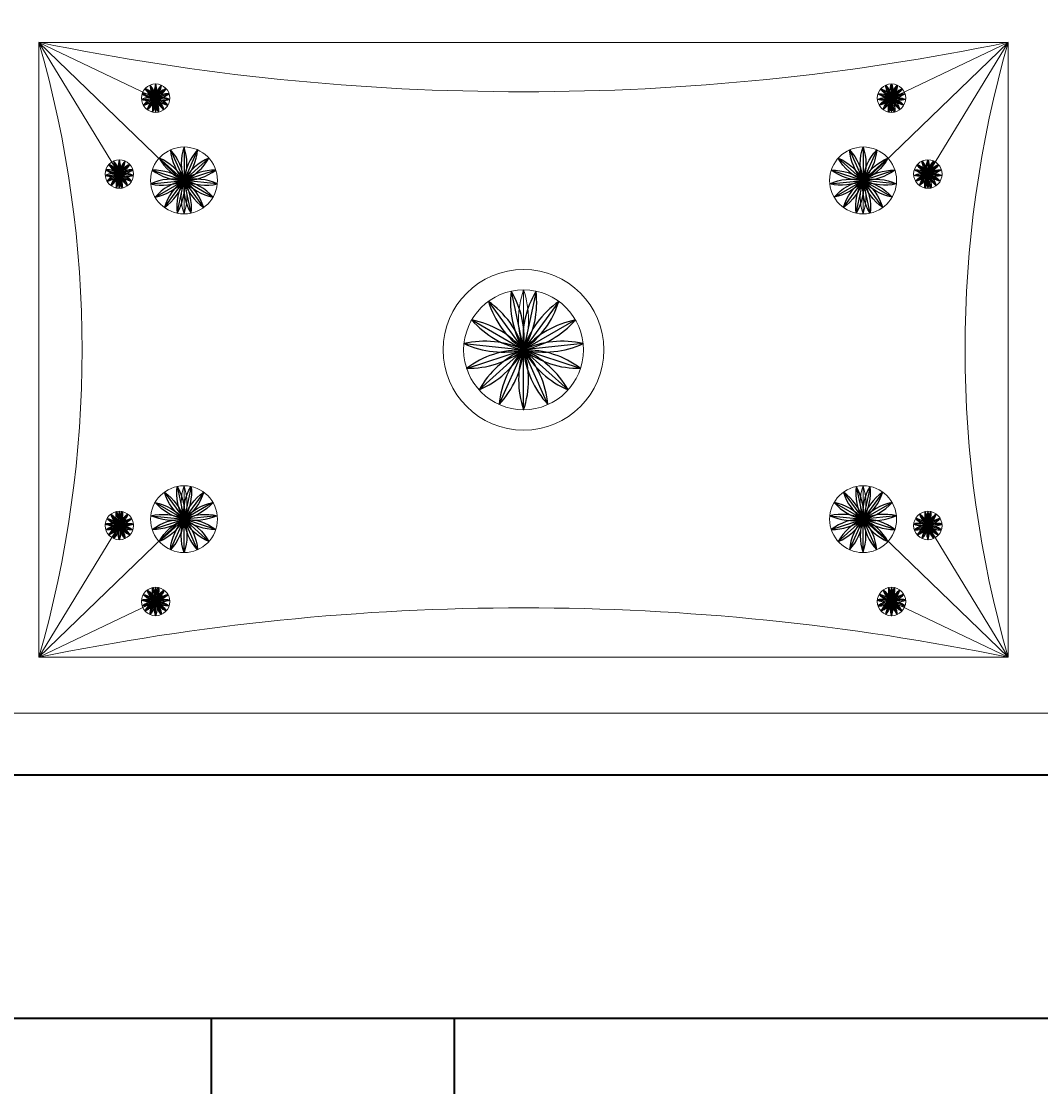
# Model space of a CAD drawing. Units: inches. Extents: x -61 to 1599, y -1316 to 257.
# Tile 34 of 204: x 109 to 134, y -790 to -763. Entities that reach past the tile are written whole.
import ezdxf

# ---------------------------------------------------------------- set-up
doc = ezdxf.new("R2010")
doc.units = ezdxf.units.IN
doc.header["$MEASUREMENT"] = 0
for name, color, linetype, lineweight in [('A-ANNO-DIMS', 2, 'Continuous', 18), ('FURNITURE', 83, 'Continuous', 18), ('WALLS', 4, 'Continuous', 35)]:
    doc.layers.add(name, color=color, linetype=linetype, lineweight=lineweight)
doc.layers.add('LT', color=8, linetype='Continuous')
doc.styles.get("Standard").update_dxf_attribs({"font": 'arial.ttf'})
doc.dimstyles.get("Standard").update_dxf_attribs({"dimtxt": 0.18, "dimasz": 0.18, "dimexe": 0.18, "dimexo": 0.0625, "dimgap": 0.09, "dimtad": 0, "dimtih": 1, "dimtoh": 1, "dimdec": 0, "dimzin": 0, "dimdsep": 46, "dimlunit": 3, "dimtxsty": 'Standard', "dimcen": 0.09, "dimadec": 0, "dimazin": 0, "dimtfac": 1, "dimtdec": 0, "dimtofl": 0, "dimtmove": 0, "dimatfit": 3, "dimfxl": 1, "dimtolj": 1, "dimtzin": 0, "dimarcsym": 0})

# ---------------------------------------------------------------- blocks, each defined once
blk = doc.blocks.new('*U15')
at = {"layer": 'LT'}
blk.add_line((0, 0.175), (0, -0.175), dxfattribs=at)
for centre, start, end in [((0.509, 0), 160.9983, 199.0017), ((-0.509, 0), 340.9983, 19.0017)]:
    blk.add_arc(centre, 0.539, start, end, dxfattribs=at)
blk = doc.blocks.new('*U16')
at = {"layer": 'LT', "transparency": 16777216}
for p, rotation in [((-66.605, -18.692), 48.00000000000001), ((-66.546, -18.649), 24), ((-66.404, -18.649), 336.0000000000001), ((-66.345, -18.692), 312), ((-66.649, -18.828), 96), ((-66.642, -18.755), 72), ((-66.627, -18.897), 120), ((-66.578, -18.951), 144), ((-66.512, -18.981), 168.0000000000001), ((-66.439, -18.981), 192), ((-66.372, -18.951), 216), ((-66.323, -18.897), 240), ((-66.308, -18.755), 288.0000000000001), ((-66.301, -18.828), 264)]:
    blk.add_blockref('*U15', p, dxfattribs=dict(at, rotation=rotation))
blk.add_blockref('*U15', (-66.475, -18.634), dxfattribs=at)
blk = doc.blocks.new('*U45')
at = {"layer": 'LT'}
blk.add_line((0, 0.175), (0, -0.175), dxfattribs=at)
for centre, start, end in [((0.509, 0), 160.9983, 199.0017), ((-0.509, 0), 340.9983, 19.0017)]:
    blk.add_arc(centre, 0.539, start, end, dxfattribs=at)
blk = doc.blocks.new('*U46')
at = {"layer": 'LT', "transparency": 16777216}
for p, rotation in [((-66.605, -18.692), 48.00000000000001), ((-66.546, -18.649), 24), ((-66.404, -18.649), 336.0000000000001), ((-66.345, -18.692), 312), ((-66.649, -18.828), 96), ((-66.642, -18.755), 72), ((-66.627, -18.897), 120), ((-66.578, -18.951), 144), ((-66.512, -18.981), 168.0000000000001), ((-66.439, -18.981), 192), ((-66.372, -18.951), 216), ((-66.323, -18.897), 240), ((-66.308, -18.755), 288.0000000000001), ((-66.301, -18.828), 264)]:
    blk.add_blockref('*U45', p, dxfattribs=dict(at, rotation=rotation))
blk.add_blockref('*U45', (-66.475, -18.634), dxfattribs=at)
blk = doc.blocks.new('*U9')
at = {"layer": 'LT'}
blk.add_line((0, 0.175), (0, -0.175), dxfattribs=at)
for centre, start, end in [((0.509, 0), 160.9983, 199.0017), ((-0.509, 0), 340.9983, 19.0017)]:
    blk.add_arc(centre, 0.539, start, end, dxfattribs=at)
blk = doc.blocks.new('*U10')
at = {"layer": 'LT', "transparency": 16777216}
for p, rotation in [((-66.605, -18.692), 48.00000000000001), ((-66.546, -18.649), 24), ((-66.404, -18.649), 336.0000000000001), ((-66.345, -18.692), 312), ((-66.649, -18.828), 96), ((-66.642, -18.755), 72), ((-66.627, -18.897), 120), ((-66.578, -18.951), 144), ((-66.512, -18.981), 168.0000000000001), ((-66.439, -18.981), 192), ((-66.372, -18.951), 216), ((-66.323, -18.897), 240), ((-66.308, -18.755), 288.0000000000001), ((-66.301, -18.828), 264)]:
    blk.add_blockref('*U9', p, dxfattribs=dict(at, rotation=rotation))
blk.add_blockref('*U9', (-66.475, -18.634), dxfattribs=at)
blk = doc.blocks.new('*U39')
at = {"layer": 'LT'}
blk.add_line((0, 0.175), (0, -0.175), dxfattribs=at)
for centre, start, end in [((0.509, 0), 160.9983, 199.0017), ((-0.509, 0), 340.9983, 19.0017)]:
    blk.add_arc(centre, 0.539, start, end, dxfattribs=at)
blk = doc.blocks.new('*U40')
at = {"layer": 'LT', "transparency": 16777216}
for p, rotation in [((-66.605, -18.692), 48.00000000000001), ((-66.546, -18.649), 24), ((-66.404, -18.649), 336.0000000000001), ((-66.345, -18.692), 312), ((-66.649, -18.828), 96), ((-66.642, -18.755), 72), ((-66.627, -18.897), 120), ((-66.578, -18.951), 144), ((-66.512, -18.981), 168.0000000000001), ((-66.439, -18.981), 192), ((-66.372, -18.951), 216), ((-66.323, -18.897), 240), ((-66.308, -18.755), 288.0000000000001), ((-66.301, -18.828), 264)]:
    blk.add_blockref('*U39', p, dxfattribs=dict(at, rotation=rotation))
blk.add_blockref('*U39', (-66.475, -18.634), dxfattribs=at)
blk = doc.blocks.new('*U17')
at = {"layer": 'LT'}
blk.add_line((0, 0.412), (0, -0.412), dxfattribs=at)
for centre, start, end in [((1.198, 0), 160.9983, 199.0017), ((-1.198, 0), 340.9983, 19.0017)]:
    blk.add_arc(centre, 1.267, start, end, dxfattribs=at)
blk = doc.blocks.new('*U18')
at = {"layer": 'LT', "transparency": 16777216}
for p, rotation in [((-156.639, -43.959), 48.00000000000001), ((-156.501, -43.858), 24), ((-156.165, -43.858), 336.0000000000001), ((-156.027, -43.959), 312), ((-156.743, -44.278), 96), ((-156.725, -44.108), 72), ((-156.69, -44.441), 120), ((-155.976, -44.441), 240), ((-155.941, -44.108), 288.0000000000001), ((-155.923, -44.278), 264), ((-156.575, -44.569), 144), ((-156.419, -44.639), 168), ((-156.247, -44.639), 192), ((-156.091, -44.569), 216)]:
    blk.add_blockref('*U17', p, dxfattribs=dict(at, rotation=rotation))
blk.add_blockref('*U17', (-156.333, -43.823), dxfattribs=at)
blk = doc.blocks.new('*U33')
at = {"layer": 'LT'}
blk.add_line((0, 0.412), (0, -0.412), dxfattribs=at)
for centre, start, end in [((1.198, 0), 160.9983, 199.0017), ((-1.198, 0), 340.9983, 19.0017)]:
    blk.add_arc(centre, 1.267, start, end, dxfattribs=at)
blk = doc.blocks.new('*U34')
at = {"layer": 'LT', "transparency": 16777216}
for p, rotation in [((-156.639, -43.959), 48.00000000000001), ((-156.501, -43.858), 24), ((-156.165, -43.858), 336.0000000000001), ((-156.027, -43.959), 312), ((-156.743, -44.278), 96), ((-156.725, -44.108), 72), ((-156.69, -44.441), 120), ((-155.976, -44.441), 240), ((-155.941, -44.108), 288.0000000000001), ((-155.923, -44.278), 264), ((-156.575, -44.569), 144), ((-156.419, -44.639), 168), ((-156.247, -44.639), 192), ((-156.091, -44.569), 216)]:
    blk.add_blockref('*U33', p, dxfattribs=dict(at, rotation=rotation))
blk.add_blockref('*U33', (-156.333, -43.823), dxfattribs=at)
blk = doc.blocks.new('*U11')
at = {"layer": 'LT'}
blk.add_line((0, 0.739), (0, -0.739), dxfattribs=at)
for centre, start, end in [((2.147, 0), 160.9983, 199.0017), ((-2.147, 0), 340.9983, 19.0017)]:
    blk.add_arc(centre, 2.27, start, end, dxfattribs=at)
blk = doc.blocks.new('*U12')
at = {"layer": 'LT', "transparency": 16777216}
blk.add_blockref('*U11', (-280.242, -78.557), dxfattribs=at)
for p, rotation in [((-280.542, -78.621), 23.99999999999999), ((-279.941, -78.621), 336.0000000000001), ((-280.791, -78.801), 48.00000000000001), ((-279.692, -78.801), 312), ((-280.945, -79.067), 72), ((-279.539, -79.067), 288.0000000000001), ((-280.977, -79.373), 96), ((-280.882, -79.665), 120), ((-280.676, -79.894), 144), ((-280.395, -80.019), 168), ((-280.088, -80.019), 191.9999999999999), ((-279.807, -79.894), 216), ((-279.602, -79.665), 240), ((-279.507, -79.373), 264)]:
    blk.add_blockref('*U11', p, dxfattribs=dict(at, rotation=rotation))
blk = doc.blocks.new('*U28')
at = {"layer": 'LT'}
blk.add_line((0, 0.412), (0, -0.412), dxfattribs=at)
for centre, start, end in [((1.198, 0), 160.9983, 199.0017), ((-1.198, 0), 340.9983, 19.0017)]:
    blk.add_arc(centre, 1.267, start, end, dxfattribs=at)
blk = doc.blocks.new('*U44')
at = {"layer": 'LT', "transparency": 16777216}
for p, rotation in [((-156.639, -43.959), 48.00000000000001), ((-156.501, -43.858), 24), ((-156.165, -43.858), 336.0000000000001), ((-156.027, -43.959), 312), ((-156.743, -44.278), 96), ((-156.725, -44.108), 72), ((-156.69, -44.441), 120), ((-155.976, -44.441), 240), ((-155.941, -44.108), 288.0000000000001), ((-155.923, -44.278), 264), ((-156.575, -44.569), 144), ((-156.419, -44.639), 168), ((-156.247, -44.639), 192), ((-156.091, -44.569), 216)]:
    blk.add_blockref('*U28', p, dxfattribs=dict(at, rotation=rotation))
blk.add_blockref('*U28', (-156.333, -43.823), dxfattribs=at)
blk = doc.blocks.new('*U13')
at = {"layer": 'LT'}
blk.add_line((0, 0.412), (0, -0.412), dxfattribs=at)
for centre, start, end in [((1.198, 0), 160.9983, 199.0017), ((-1.198, 0), 340.9983, 19.0017)]:
    blk.add_arc(centre, 1.267, start, end, dxfattribs=at)
blk = doc.blocks.new('*U14')
at = {"layer": 'LT', "transparency": 16777216}
for p, rotation in [((-156.639, -43.959), 48.00000000000001), ((-156.501, -43.858), 24), ((-156.165, -43.858), 336.0000000000001), ((-156.027, -43.959), 312), ((-156.743, -44.278), 96), ((-156.725, -44.108), 72), ((-156.69, -44.441), 120), ((-155.976, -44.441), 240), ((-155.941, -44.108), 288.0000000000001), ((-155.923, -44.278), 264), ((-156.575, -44.569), 144), ((-156.419, -44.639), 168), ((-156.247, -44.639), 192), ((-156.091, -44.569), 216)]:
    blk.add_blockref('*U13', p, dxfattribs=dict(at, rotation=rotation))
blk.add_blockref('*U13', (-156.333, -43.823), dxfattribs=at)
blk = doc.blocks.new('*U19')
at = {"layer": 'LT'}
blk.add_line((0, 0.175), (0, -0.175), dxfattribs=at)
for centre, start, end in [((0.509, 0), 160.9983, 199.0017), ((-0.509, 0), 340.9983, 19.0017)]:
    blk.add_arc(centre, 0.539, start, end, dxfattribs=at)
blk = doc.blocks.new('*U6')
at = {"layer": 'LT', "transparency": 16777216}
for p, rotation in [((-66.605, -18.692), 48.00000000000001), ((-66.546, -18.649), 24), ((-66.404, -18.649), 336.0000000000001), ((-66.345, -18.692), 312), ((-66.649, -18.828), 96), ((-66.642, -18.755), 72), ((-66.627, -18.897), 120), ((-66.578, -18.951), 144), ((-66.512, -18.981), 168.0000000000001), ((-66.439, -18.981), 192), ((-66.372, -18.951), 216), ((-66.323, -18.897), 240), ((-66.308, -18.755), 288.0000000000001), ((-66.301, -18.828), 264)]:
    blk.add_blockref('*U19', p, dxfattribs=dict(at, rotation=rotation))
blk.add_blockref('*U19', (-66.475, -18.634), dxfattribs=at)
blk = doc.blocks.new('*U35')
at = {"layer": 'LT'}
blk.add_line((0, 0.175), (0, -0.175), dxfattribs=at)
for centre, start, end in [((0.509, 0), 160.9983, 199.0017), ((-0.509, 0), 340.9983, 19.0017)]:
    blk.add_arc(centre, 0.539, start, end, dxfattribs=at)
blk = doc.blocks.new('*U36')
at = {"layer": 'LT', "transparency": 16777216}
for p, rotation in [((-66.605, -18.692), 48.00000000000001), ((-66.546, -18.649), 24), ((-66.404, -18.649), 336.0000000000001), ((-66.345, -18.692), 312), ((-66.649, -18.828), 96), ((-66.642, -18.755), 72), ((-66.627, -18.897), 120), ((-66.578, -18.951), 144), ((-66.512, -18.981), 168.0000000000001), ((-66.439, -18.981), 192), ((-66.372, -18.951), 216), ((-66.323, -18.897), 240), ((-66.308, -18.755), 288.0000000000001), ((-66.301, -18.828), 264)]:
    blk.add_blockref('*U35', p, dxfattribs=dict(at, rotation=rotation))
blk.add_blockref('*U35', (-66.475, -18.634), dxfattribs=at)
blk = doc.blocks.new('*U7')
at = {"layer": 'LT'}
blk.add_line((0, 0.175), (0, -0.175), dxfattribs=at)
for centre, start, end in [((0.509, 0), 160.9983, 199.0017), ((-0.509, 0), 340.9983, 19.0017)]:
    blk.add_arc(centre, 0.539, start, end, dxfattribs=at)
blk = doc.blocks.new('*U8')
at = {"layer": 'LT', "transparency": 16777216}
for p, rotation in [((-66.605, -18.692), 48.00000000000001), ((-66.546, -18.649), 24), ((-66.404, -18.649), 336.0000000000001), ((-66.345, -18.692), 312), ((-66.649, -18.828), 96), ((-66.642, -18.755), 72), ((-66.627, -18.897), 120), ((-66.578, -18.951), 144), ((-66.512, -18.981), 168.0000000000001), ((-66.439, -18.981), 192), ((-66.372, -18.951), 216), ((-66.323, -18.897), 240), ((-66.308, -18.755), 288.0000000000001), ((-66.301, -18.828), 264)]:
    blk.add_blockref('*U7', p, dxfattribs=dict(at, rotation=rotation))
blk.add_blockref('*U7', (-66.475, -18.634), dxfattribs=at)
blk = doc.blocks.new('*U37')
at = {"layer": 'LT'}
blk.add_line((0, 0.175), (0, -0.175), dxfattribs=at)
for centre, start, end in [((0.509, 0), 160.9983, 199.0017), ((-0.509, 0), 340.9983, 19.0017)]:
    blk.add_arc(centre, 0.539, start, end, dxfattribs=at)
blk = doc.blocks.new('*U38')
at = {"layer": 'LT', "transparency": 16777216}
for p, rotation in [((-66.605, -18.692), 48.00000000000001), ((-66.546, -18.649), 24), ((-66.404, -18.649), 336.0000000000001), ((-66.345, -18.692), 312), ((-66.649, -18.828), 96), ((-66.642, -18.755), 72), ((-66.627, -18.897), 120), ((-66.578, -18.951), 144), ((-66.512, -18.981), 168.0000000000001), ((-66.439, -18.981), 192), ((-66.372, -18.951), 216), ((-66.323, -18.897), 240), ((-66.308, -18.755), 288.0000000000001), ((-66.301, -18.828), 264)]:
    blk.add_blockref('*U37', p, dxfattribs=dict(at, rotation=rotation))
blk.add_blockref('*U37', (-66.475, -18.634), dxfattribs=at)
blk = doc.blocks.new('BED-DOUBLE')
for p, q in [((10.471, 1.379), (10.471, 16.557)), ((34.388, 16.557), (10.471, 16.557)), ((10.471, 16.557), (13.35, 15.18)), ((10.471, 16.557), (14.039, 13.107)), ((10.471, 16.557), (12.454, 13.305)), ((34.388, 16.557), (30.82, 13.107)), ((34.388, 16.557), (31.508, 15.18)), ((34.388, 16.557), (32.405, 13.305)), ((13.35, 15.18), (13.35, 14.829)), ((31.508, 15.18), (31.508, 14.829)), ((12.454, 13.305), (12.454, 12.955)), ((14.052, 13.149), (14.052, 12.324)), ((30.806, 13.149), (30.806, 12.324)), ((32.405, 13.305), (32.405, 12.955)), ((22.429, 8.968), (22.429, 10.447)), ((14.052, 4.788), (14.052, 5.613)), ((30.806, 4.788), (30.806, 5.613)), ((10.471, 1.379), (14.039, 4.83)), ((12.454, 4.631), (12.454, 4.982)), ((34.388, 1.379), (30.82, 4.83)), ((32.405, 4.631), (32.405, 4.982)), ((10.471, 1.379), (12.454, 4.631)), ((34.388, 1.379), (32.405, 4.631)), ((13.35, 2.756), (13.35, 3.107)), ((31.508, 2.756), (31.508, 3.107)), ((10.471, 1.379), (13.35, 2.756)), ((34.388, 1.379), (31.508, 2.756)), ((34.388, 1.379), (34.388, 1.379))]:
    blk.add_line(p, q)
for points in [[(1.272, 88.537), (1.272, 3.449, 0.414214), (4.722, 0), (66.813, 0, 0.414214), (70.263, 3.449), (70.263, 88.537, 0.414214), (66.813, 91.987), (4.722, 91.987, 0.414214)], [(13.35, 15.18, 0.167358), (13.35, 14.829, 0.167358)], [(12.454, 13.305, 0.167358), (12.454, 12.955, 0.167358)], [(14.052, 13.149, 0.167358), (14.052, 12.324, 0.167358)], [(30.806, 12.324, 0.167358), (30.806, 13.149, 0.167358)], [(32.405, 12.955, 0.167358), (32.405, 13.305, 0.167358)], [(22.429, 8.968, 0.167358), (22.429, 10.447, 0.167358)], [(14.052, 5.613, 0.167358), (14.052, 4.788, 0.167358)], [(30.806, 4.788, 0.167358), (30.806, 5.613, 0.167358)], [(12.454, 4.982, 0.167358), (12.454, 4.631, 0.167358)], [(32.405, 4.631, 0.167358), (32.405, 4.982, 0.167358)], [(13.35, 3.107, 0.167358), (13.35, 2.756, 0.167358)], [(31.508, 2.756, 0.167358), (31.508, 3.107, 0.167358)]]:
    blk.add_lwpolyline(points, format="xyb", close=True)
blk.add_lwpolyline([(34.388, 16.557), (34.388, 1.379), (10.471, 1.379), (10.471, 16.557), (34.388, 16.557), (34.388, 1.379), (10.471, 1.379)])
for centre, radius in [((13.35, 15.18), 0.351), ((31.508, 15.18), 0.351), ((14.052, 13.149), 0.825), ((30.806, 13.149), 0.825), ((12.454, 13.305), 0.351), ((32.405, 13.305), 0.351), ((22.429, 8.968), 1.982), ((22.429, 8.968), 1.478), ((14.052, 4.788), 0.825), ((30.806, 4.788), 0.825), ((12.454, 4.631), 0.351), ((32.405, 4.631), 0.351), ((13.35, 2.756), 0.351), ((31.508, 2.756), 0.351)]:
    blk.add_circle(centre, radius)
for centre, radius, start, end in [((-16.003, 8.968), 27.54, 344.0046, 15.9954), ((22.429, 74.54), 59.203, 258.34678, 281.65322), ((60.861, 8.968), 27.54, 164.0046, 195.9954), ((32.017, 15.005), 0.539, 160.9983, 199.0017), ((30.999, 15.005), 0.539, 340.9983, 19.0017), ((22.429, -56.603), 59.203, 78.34678, 101.65322)]:
    blk.add_arc(centre, radius, start, end)
for name, p in [('*U40', (79.825, 33.99)), ('*U34', (170.385, 57.384)), ('*U46', (78.929, 32.115))]:
    blk.add_blockref(name, p)
at = {"extrusion": (0, 0, -1), "zscale": -1}
for name, p in [('*U36', (34.967, 33.99)), ('*U14', (125.527, 57.384)), ('*U38', (34.07, 32.115))]:
    blk.add_blockref(name, p, dxfattribs=at)
at = {"rotation": 180}
for name, p in [('*U12', (-257.812, -70.328)), ('*U44', (-125.527, -39.447)), ('*U8', (-34.07, -14.178)), ('*U6', (-34.967, -16.053))]:
    blk.add_blockref(name, p, dxfattribs=at)
at = {"extrusion": (0, 0, -1), "zscale": -1, "rotation": 180}
for name, p in [('*U18', (-170.385, -39.447)), ('*U16', (-78.929, -14.178)), ('*U10', (-79.825, -16.053))]:
    blk.add_blockref(name, p, dxfattribs=at)
blk = doc.blocks.new('*D687')
at = {"layer": 'A-ANNO-DIMS', "color": 0, "lineweight": -2, "transparency": 16777216}
for p, q in [((289.418, 181.677), (-61.077, 181.677)), ((-60.897, 181.497), (-60.897, -528.952)), ((-60.897, -1239.765), (-60.897, -529.316)), ((319.64, -1239.945), (-61.077, -1239.945))]:
    blk.add_line(p, q, dxfattribs=at)
at = {"layer": 'A-ANNO-DIMS', "color": 0, "transparency": 16777216}
for points in [[(-60.927, 181.497), (-60.867, 181.497), (-60.897, 181.677)], [(-60.927, -1239.765), (-60.867, -1239.765), (-60.897, -1239.945)]]:
    blk.add_solid(points, dxfattribs=at)
at = {"layer": 'DEFPOINTS', "color": 0, "transparency": 16777216}
for p in [(289.481, 181.677), (-60.897, -1239.945), (319.703, -1239.945)]:
    blk.add_point(p, dxfattribs=at)
at = {"layer": 'A-ANNO-DIMS', "color": 0, "transparency": 16777216, "insert": (-60.897, -529.134), "char_height": 0.18, "attachment_point": 5}
blk.add_mtext('\\A1;1421.6', dxfattribs=at)

msp = doc.modelspace()

# ---------------------------------------------------------------- linework, layer by layer
at = {"layer": 'WALLS'}
for p, q in [((14.7028, -781.9446), (237.7028, -781.9446)), ((14.7028, -787.9446), (237.7028, -787.9446)), ((113.7028, -943.9446), (113.7028, -787.9446)), ((119.7028, -943.9446), (119.7028, -787.9446))]:
    msp.add_line(p, q, dxfattribs=at)

# ---------------------------------------------------------------- block references
at = {"layer": 'FURNITURE'}
msp.add_blockref('BED-DOUBLE', (98.977, -780.4187), dxfattribs=at)

# ---------------------------------------------------------------- dimensions: what is measured, and where the dimension line sits
at = {"layer": 'A-ANNO-DIMS'}
dim = msp.add_linear_dim(base=(-60.8972, -1239.9446), p1=(289.4807, 181.6771), p2=(319.7028, -1239.9446), angle=90, dimstyle='Standard', override={"dimdec": 1, "dimlfac": 1, "dimrnd": 0, "dimzin": 0, "dimdsep": 46, "dimlunit": 2}, dxfattribs=at)
dim.commit()
dim.dimension.update_dxf_attribs({"geometry": '*D687', "text_midpoint": (-60.8972, -529.1337)})

doc.saveas('drawing.dxf')
